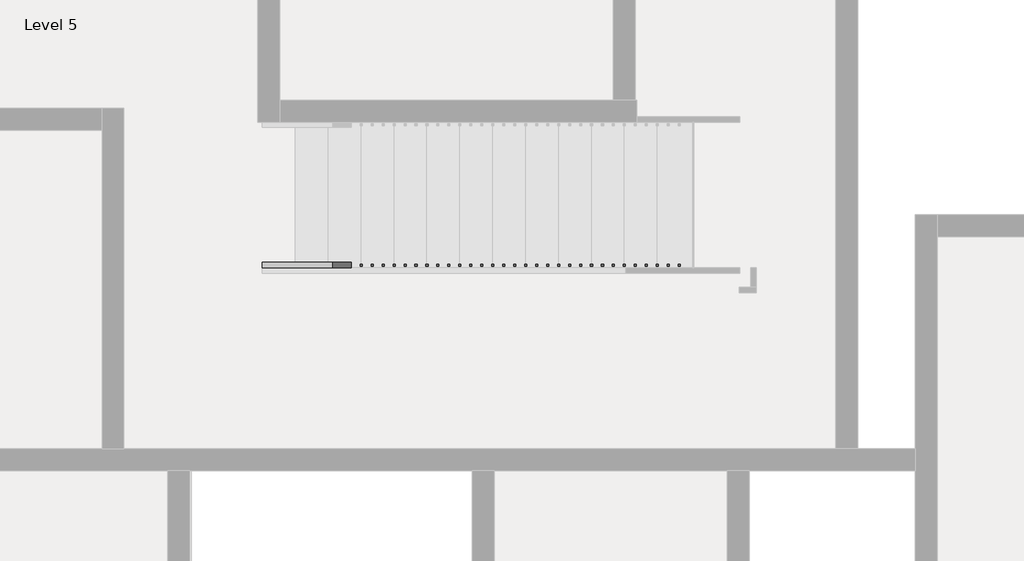
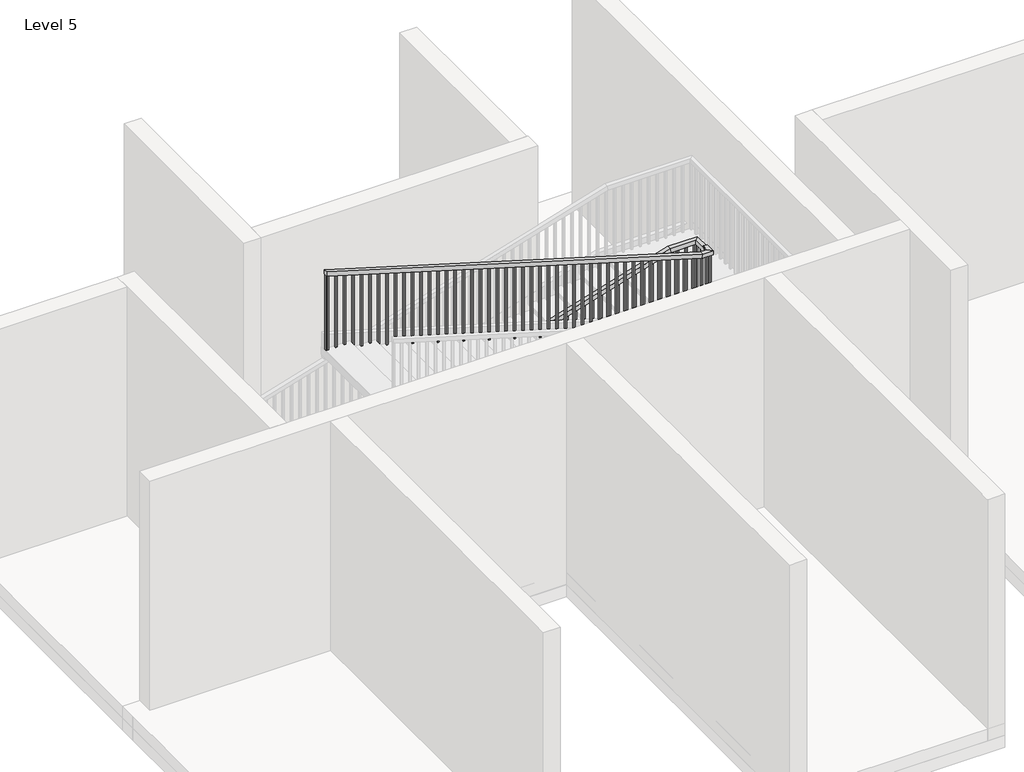
# One storey, part 11 of 14: 1 railing.
"""IFC4 building model written with IfcOpenShell, lengths in millimetres."""

from ifc_helpers import new_model, si_unit, frame, origin, place, context, project, spatial, polyline, outline, extrude, faceted_brep, element, save

model = new_model("IFC4")

# Units and contexts
model_context = context("Model", 3, world=origin())
ifc_project = project(units=[si_unit("LENGTHUNIT", "METRE", prefix="MILLI")], contexts=[model_context])

# Site, building, storey
site = spatial("IfcSite", under=ifc_project)
building = spatial("IfcBuilding", under=site)
storey = spatial("IfcBuildingStorey", under=building, Name="Level 5", Elevation=12192.0)

# Railing
placement = place(None, origin())
element("IfcRailing", 1, ObjectType="Handrail - Rectangular", at=placement, inside=storey, context=model_context, shape_type="SolidModel", body=[
    faceted_brep([(-5254.0891351, 11205.0082924, 13197.84), (-5254.0891351, 11205.0082924, 13144.8032429), (-5254.0891351, 11154.2082924, 13144.8032429), (-5254.0891351, 11154.2082924, 13197.84), (-986.8891351, 11205.0082924, 14478.0), (-979.4332782, 11205.0082924, 14427.2), (-979.4332782, 11154.2082924, 14427.2), (-986.8891351, 11154.2082924, 14478.0), (-631.2891351, 11205.0082924, 14478.0), (-631.2891351, 11205.0082924, 14427.2), (-682.0891351, 11154.2082924, 14427.2), (-682.0891351, 11154.2082924, 14478.0), (-631.2891351, 11001.8082924, 14478.0), (-631.2891351, 10951.0082924, 14427.2), (-682.0891351, 10951.0082924, 14427.2), (-682.0891351, 11001.8082924, 14478.0), (-631.2891351, 11001.8082924, 14500.86), (-631.2891351, 10951.0082924, 14450.06), (-682.0891351, 10951.0082924, 14450.06), (-682.0891351, 11001.8082924, 14500.86), (-631.2891351, 10874.8082924, 14500.86), (-631.2891351, 10874.8082924, 14450.06), (-682.0891351, 10925.6082924, 14450.06), (-682.0891351, 10925.6082924, 14500.86), (-758.2891351, 10874.8082924, 14500.86), (-765.744992, 10874.8082924, 14450.06), (-765.744992, 10925.6082924, 14450.06), (-758.2891351, 10925.6082924, 14500.86), (-5254.0891351, 10874.8082924, 15849.6), (-5254.0891351, 10925.6082924, 15849.6), (-5254.0891351, 10925.6082924, 15796.5632429), (-5254.0891351, 10874.8082924, 15796.5632429)], [[[0, 1, 2, 3]], [[1, 0, 4, 5]], [[2, 1, 5, 6]], [[3, 2, 6, 7]], [[0, 3, 7, 4]], [[5, 4, 8, 9]], [[6, 5, 9, 10]], [[7, 6, 10, 11]], [[4, 7, 11, 8]], [[9, 8, 12, 13]], [[10, 9, 13, 14]], [[11, 10, 14, 15]], [[8, 11, 15, 12]], [[13, 12, 16, 17]], [[14, 13, 17, 18]], [[15, 14, 18, 19]], [[12, 15, 19, 16]], [[17, 16, 20, 21]], [[18, 17, 21, 22]], [[19, 18, 22, 23]], [[16, 19, 23, 20]], [[21, 20, 24, 25]], [[22, 21, 25, 26]], [[23, 22, 26, 27]], [[20, 23, 27, 24]], [[28, 29, 30, 31]], [[25, 24, 28, 31]], [[26, 25, 31, 30]], [[27, 26, 30, 29]], [[24, 27, 29, 28]]]),
    extrude(outline(polyline([(15786.0857429, -5219.1641351), (15791.8007429, -5238.2141351), (14843.76, -5238.2141351), (14843.76, -5219.1641351), (15786.0857429, -5219.1641351)])), frame((0.0, 10890.6832924, 0.0), z_axis=(0.0, 1.0, 0.0), x_axis=(0.0, 0.0, 1.0)), (0.0, 0.0, 1.0), 19.05),
    extrude(outline(polyline([(15755.6057429, -5117.5641351), (15761.3207429, -5136.6141351), (14843.76, -5136.6141351), (14843.76, -5117.5641351), (15755.6057429, -5117.5641351)])), frame((0.0, 10890.6832924, 0.0), z_axis=(0.0, 1.0, 0.0), x_axis=(0.0, 0.0, 1.0)), (0.0, 0.0, 1.0), 19.05),
    extrude(outline(polyline([(15725.1257429, -5015.9641351), (15730.8407429, -5035.0141351), (14843.76, -5035.0141351), (14843.76, -5015.9641351), (15725.1257429, -5015.9641351)])), frame((0.0, 10890.6832924, 0.0), z_axis=(0.0, 1.0, 0.0), x_axis=(0.0, 0.0, 1.0)), (0.0, 0.0, 1.0), 19.05),
    extrude(outline(polyline([(15694.6457429, -4914.3641351), (15700.3607429, -4933.4141351), (14752.32, -4933.4141351), (14752.32, -4914.3641351), (15694.6457429, -4914.3641351)])), frame((0.0, 10890.6832924, 0.0), z_axis=(0.0, 1.0, 0.0), x_axis=(0.0, 0.0, 1.0)), (0.0, 0.0, 1.0), 19.05),
    extrude(outline(polyline([(15664.1657429, -4812.7641351), (15669.8807429, -4831.8141351), (14752.32, -4831.8141351), (14752.32, -4812.7641351), (15664.1657429, -4812.7641351)])), frame((0.0, 10890.6832924, 0.0), z_axis=(0.0, 1.0, 0.0), x_axis=(0.0, 0.0, 1.0)), (0.0, 0.0, 1.0), 19.05),
    extrude(outline(polyline([(15633.6857429, -4711.1641351), (15639.4007429, -4730.2141351), (14752.32, -4730.2141351), (14752.32, -4711.1641351), (15633.6857429, -4711.1641351)])), frame((0.0, 10890.6832924, 0.0), z_axis=(0.0, 1.0, 0.0), x_axis=(0.0, 0.0, 1.0)), (0.0, 0.0, 1.0), 19.05),
    extrude(outline(polyline([(15603.2057429, -4609.5641351), (15608.9207429, -4628.6141351), (14660.88, -4628.6141351), (14660.88, -4609.5641351), (15603.2057429, -4609.5641351)])), frame((0.0, 10890.6832924, 0.0), z_axis=(0.0, 1.0, 0.0), x_axis=(0.0, 0.0, 1.0)), (0.0, 0.0, 1.0), 19.05),
    extrude(outline(polyline([(15572.7257429, -4507.9641351), (15578.4407429, -4527.0141351), (14660.88, -4527.0141351), (14660.88, -4507.9641351), (15572.7257429, -4507.9641351)])), frame((0.0, 10890.6832924, 0.0), z_axis=(0.0, 1.0, 0.0), x_axis=(0.0, 0.0, 1.0)), (0.0, 0.0, 1.0), 19.05),
    extrude(outline(polyline([(15542.2457429, -4406.3641351), (15547.9607429, -4425.4141351), (14660.88, -4425.4141351), (14660.88, -4406.3641351), (15542.2457429, -4406.3641351)])), frame((0.0, 10890.6832924, 0.0), z_axis=(0.0, 1.0, 0.0), x_axis=(0.0, 0.0, 1.0)), (0.0, 0.0, 1.0), 19.05),
    extrude(outline(polyline([(15511.7657429, -4304.7641351), (15517.4807429, -4323.8141351), (14569.44, -4323.8141351), (14569.44, -4304.7641351), (15511.7657429, -4304.7641351)])), frame((0.0, 10890.6832924, 0.0), z_axis=(0.0, 1.0, 0.0), x_axis=(0.0, 0.0, 1.0)), (0.0, 0.0, 1.0), 19.05),
    extrude(outline(polyline([(15481.2857429, -4203.1641351), (15487.0007429, -4222.2141351), (14569.44, -4222.2141351), (14569.44, -4203.1641351), (15481.2857429, -4203.1641351)])), frame((0.0, 10890.6832924, 0.0), z_axis=(0.0, 1.0, 0.0), x_axis=(0.0, 0.0, 1.0)), (0.0, 0.0, 1.0), 19.05),
    extrude(outline(polyline([(15450.8057429, -4101.5641351), (15456.5207429, -4120.6141351), (14569.44, -4120.6141351), (14569.44, -4101.5641351), (15450.8057429, -4101.5641351)])), frame((0.0, 10890.6832924, 0.0), z_axis=(0.0, 1.0, 0.0), x_axis=(0.0, 0.0, 1.0)), (0.0, 0.0, 1.0), 19.05),
    extrude(outline(polyline([(15420.3257429, -3999.9641351), (15426.0407429, -4019.0141351), (14478.0, -4019.0141351), (14478.0, -3999.9641351), (15420.3257429, -3999.9641351)])), frame((0.0, 10890.6832924, 0.0), z_axis=(0.0, 1.0, 0.0), x_axis=(0.0, 0.0, 1.0)), (0.0, 0.0, 1.0), 19.05),
    extrude(outline(polyline([(15389.8457429, -3898.3641351), (15395.5607429, -3917.4141351), (14478.0, -3917.4141351), (14478.0, -3898.3641351), (15389.8457429, -3898.3641351)])), frame((0.0, 10890.6832924, 0.0), z_axis=(0.0, 1.0, 0.0), x_axis=(0.0, 0.0, 1.0)), (0.0, 0.0, 1.0), 19.05),
    extrude(outline(polyline([(15359.3657429, -3796.7641351), (15365.0807429, -3815.8141351), (14478.0, -3815.8141351), (14478.0, -3796.7641351), (15359.3657429, -3796.7641351)])), frame((0.0, 10890.6832924, 0.0), z_axis=(0.0, 1.0, 0.0), x_axis=(0.0, 0.0, 1.0)), (0.0, 0.0, 1.0), 19.05),
    extrude(outline(polyline([(15328.8857429, -3695.1641351), (15334.6007429, -3714.2141351), (14386.56, -3714.2141351), (14386.56, -3695.1641351), (15328.8857429, -3695.1641351)])), frame((0.0, 10890.6832924, 0.0), z_axis=(0.0, 1.0, 0.0), x_axis=(0.0, 0.0, 1.0)), (0.0, 0.0, 1.0), 19.05),
    extrude(outline(polyline([(15298.4057429, -3593.5641351), (15304.1207429, -3612.6141351), (14386.56, -3612.6141351), (14386.56, -3593.5641351), (15298.4057429, -3593.5641351)])), frame((0.0, 10890.6832924, 0.0), z_axis=(0.0, 1.0, 0.0), x_axis=(0.0, 0.0, 1.0)), (0.0, 0.0, 1.0), 19.05),
    extrude(outline(polyline([(15267.9257429, -3491.9641351), (15273.6407429, -3511.0141351), (14386.56, -3511.0141351), (14386.56, -3491.9641351), (15267.9257429, -3491.9641351)])), frame((0.0, 10890.6832924, 0.0), z_axis=(0.0, 1.0, 0.0), x_axis=(0.0, 0.0, 1.0)), (0.0, 0.0, 1.0), 19.05),
    extrude(outline(polyline([(15237.4457429, -3390.3641351), (15243.1607429, -3409.4141351), (14295.12, -3409.4141351), (14295.12, -3390.3641351), (15237.4457429, -3390.3641351)])), frame((0.0, 10890.6832924, 0.0), z_axis=(0.0, 1.0, 0.0), x_axis=(0.0, 0.0, 1.0)), (0.0, 0.0, 1.0), 19.05),
    extrude(outline(polyline([(15206.9657429, -3288.7641351), (15212.6807429, -3307.8141351), (14295.12, -3307.8141351), (14295.12, -3288.7641351), (15206.9657429, -3288.7641351)])), frame((0.0, 10890.6832924, 0.0), z_axis=(0.0, 1.0, 0.0), x_axis=(0.0, 0.0, 1.0)), (0.0, 0.0, 1.0), 19.05),
    extrude(outline(polyline([(15176.4857429, -3187.1641351), (15182.2007429, -3206.2141351), (14295.12, -3206.2141351), (14295.12, -3187.1641351), (15176.4857429, -3187.1641351)])), frame((0.0, 10890.6832924, 0.0), z_axis=(0.0, 1.0, 0.0), x_axis=(0.0, 0.0, 1.0)), (0.0, 0.0, 1.0), 19.05),
    extrude(outline(polyline([(15146.0057429, -3085.5641351), (15151.7207429, -3104.6141351), (14203.68, -3104.6141351), (14203.68, -3085.5641351), (15146.0057429, -3085.5641351)])), frame((0.0, 10890.6832924, 0.0), z_axis=(0.0, 1.0, 0.0), x_axis=(0.0, 0.0, 1.0)), (0.0, 0.0, 1.0), 19.05),
    extrude(outline(polyline([(15115.5257429, -2983.9641351), (15121.2407429, -3003.0141351), (14203.68, -3003.0141351), (14203.68, -2983.9641351), (15115.5257429, -2983.9641351)])), frame((0.0, 10890.6832924, 0.0), z_axis=(0.0, 1.0, 0.0), x_axis=(0.0, 0.0, 1.0)), (0.0, 0.0, 1.0), 19.05),
    extrude(outline(polyline([(15085.0457429, -2882.3641351), (15090.7607429, -2901.4141351), (14203.68, -2901.4141351), (14203.68, -2882.3641351), (15085.0457429, -2882.3641351)])), frame((0.0, 10890.6832924, 0.0), z_axis=(0.0, 1.0, 0.0), x_axis=(0.0, 0.0, 1.0)), (0.0, 0.0, 1.0), 19.05),
    extrude(outline(polyline([(15054.5657429, -2780.7641351), (15060.2807429, -2799.8141351), (14112.24, -2799.8141351), (14112.24, -2780.7641351), (15054.5657429, -2780.7641351)])), frame((0.0, 10890.6832924, 0.0), z_axis=(0.0, 1.0, 0.0), x_axis=(0.0, 0.0, 1.0)), (0.0, 0.0, 1.0), 19.05),
    extrude(outline(polyline([(15024.0857429, -2679.1641351), (15029.8007429, -2698.2141351), (14112.24, -2698.2141351), (14112.24, -2679.1641351), (15024.0857429, -2679.1641351)])), frame((0.0, 10890.6832924, 0.0), z_axis=(0.0, 1.0, 0.0), x_axis=(0.0, 0.0, 1.0)), (0.0, 0.0, 1.0), 19.05),
    extrude(outline(polyline([(14993.6057429, -2577.5641351), (14999.3207429, -2596.6141351), (14112.24, -2596.6141351), (14112.24, -2577.5641351), (14993.6057429, -2577.5641351)])), frame((0.0, 10890.6832924, 0.0), z_axis=(0.0, 1.0, 0.0), x_axis=(0.0, 0.0, 1.0)), (0.0, 0.0, 1.0), 19.05),
    extrude(outline(polyline([(14963.1257429, -2475.9641351), (14968.8407429, -2495.0141351), (14020.8, -2495.0141351), (14020.8, -2475.9641351), (14963.1257429, -2475.9641351)])), frame((0.0, 10890.6832924, 0.0), z_axis=(0.0, 1.0, 0.0), x_axis=(0.0, 0.0, 1.0)), (0.0, 0.0, 1.0), 19.05),
    extrude(outline(polyline([(14932.6457429, -2374.3641351), (14938.3607429, -2393.4141351), (14020.8, -2393.4141351), (14020.8, -2374.3641351), (14932.6457429, -2374.3641351)])), frame((0.0, 10890.6832924, 0.0), z_axis=(0.0, 1.0, 0.0), x_axis=(0.0, 0.0, 1.0)), (0.0, 0.0, 1.0), 19.05),
    extrude(outline(polyline([(14902.1657429, -2272.7641351), (14907.8807429, -2291.8141351), (14020.8, -2291.8141351), (14020.8, -2272.7641351), (14902.1657429, -2272.7641351)])), frame((0.0, 10890.6832924, 0.0), z_axis=(0.0, 1.0, 0.0), x_axis=(0.0, 0.0, 1.0)), (0.0, 0.0, 1.0), 19.05),
    extrude(outline(polyline([(14871.6857429, -2171.1641351), (14877.4007429, -2190.2141351), (13929.36, -2190.2141351), (13929.36, -2171.1641351), (14871.6857429, -2171.1641351)])), frame((0.0, 10890.6832924, 0.0), z_axis=(0.0, 1.0, 0.0), x_axis=(0.0, 0.0, 1.0)), (0.0, 0.0, 1.0), 19.05),
    extrude(outline(polyline([(14841.2057429, -2069.5641351), (14846.9207429, -2088.6141351), (13929.36, -2088.6141351), (13929.36, -2069.5641351), (14841.2057429, -2069.5641351)])), frame((0.0, 10890.6832924, 0.0), z_axis=(0.0, 1.0, 0.0), x_axis=(0.0, 0.0, 1.0)), (0.0, 0.0, 1.0), 19.05),
    extrude(outline(polyline([(14810.7257429, -1967.9641351), (14816.4407429, -1987.0141351), (13929.36, -1987.0141351), (13929.36, -1967.9641351), (14810.7257429, -1967.9641351)])), frame((0.0, 10890.6832924, 0.0), z_axis=(0.0, 1.0, 0.0), x_axis=(0.0, 0.0, 1.0)), (0.0, 0.0, 1.0), 19.05),
    extrude(outline(polyline([(14780.2457429, -1866.3641351), (14785.9607429, -1885.4141351), (13837.92, -1885.4141351), (13837.92, -1866.3641351), (14780.2457429, -1866.3641351)])), frame((0.0, 10890.6832924, 0.0), z_axis=(0.0, 1.0, 0.0), x_axis=(0.0, 0.0, 1.0)), (0.0, 0.0, 1.0), 19.05),
    extrude(outline(polyline([(14749.7657429, -1764.7641351), (14755.4807429, -1783.8141351), (13837.92, -1783.8141351), (13837.92, -1764.7641351), (14749.7657429, -1764.7641351)])), frame((0.0, 10890.6832924, 0.0), z_axis=(0.0, 1.0, 0.0), x_axis=(0.0, 0.0, 1.0)), (0.0, 0.0, 1.0), 19.05),
    extrude(outline(polyline([(14719.2857429, -1663.1641351), (14725.0007429, -1682.2141351), (13837.92, -1682.2141351), (13837.92, -1663.1641351), (14719.2857429, -1663.1641351)])), frame((0.0, 10890.6832924, 0.0), z_axis=(0.0, 1.0, 0.0), x_axis=(0.0, 0.0, 1.0)), (0.0, 0.0, 1.0), 19.05),
    extrude(outline(polyline([(14688.8057429, -1561.5641351), (14694.5207429, -1580.6141351), (13746.48, -1580.6141351), (13746.48, -1561.5641351), (14688.8057429, -1561.5641351)])), frame((0.0, 10890.6832924, 0.0), z_axis=(0.0, 1.0, 0.0), x_axis=(0.0, 0.0, 1.0)), (0.0, 0.0, 1.0), 19.05),
    extrude(outline(polyline([(14658.3257429, -1459.9641351), (14664.0407429, -1479.0141351), (13746.48, -1479.0141351), (13746.48, -1459.9641351), (14658.3257429, -1459.9641351)])), frame((0.0, 10890.6832924, 0.0), z_axis=(0.0, 1.0, 0.0), x_axis=(0.0, 0.0, 1.0)), (0.0, 0.0, 1.0), 19.05),
    extrude(outline(polyline([(14627.8457429, -1358.3641351), (14633.5607429, -1377.4141351), (13746.48, -1377.4141351), (13746.48, -1358.3641351), (14627.8457429, -1358.3641351)])), frame((0.0, 10890.6832924, 0.0), z_axis=(0.0, 1.0, 0.0), x_axis=(0.0, 0.0, 1.0)), (0.0, 0.0, 1.0), 19.05),
    extrude(outline(polyline([(14597.3657429, -1256.7641351), (14603.0807429, -1275.8141351), (13655.04, -1275.8141351), (13655.04, -1256.7641351), (14597.3657429, -1256.7641351)])), frame((0.0, 10890.6832924, 0.0), z_axis=(0.0, 1.0, 0.0), x_axis=(0.0, 0.0, 1.0)), (0.0, 0.0, 1.0), 19.05),
    extrude(outline(polyline([(14566.8857429, -1155.1641351), (14572.6007429, -1174.2141351), (13655.04, -1174.2141351), (13655.04, -1155.1641351), (14566.8857429, -1155.1641351)])), frame((0.0, 10890.6832924, 0.0), z_axis=(0.0, 1.0, 0.0), x_axis=(0.0, 0.0, 1.0)), (0.0, 0.0, 1.0), 19.05),
    extrude(outline(polyline([(14536.4057429, -1053.5641351), (14542.1207429, -1072.6141351), (13655.04, -1072.6141351), (13655.04, -1053.5641351), (14536.4057429, -1053.5641351)])), frame((0.0, 10890.6832924, 0.0), z_axis=(0.0, 1.0, 0.0), x_axis=(0.0, 0.0, 1.0)), (0.0, 0.0, 1.0), 19.05),
    extrude(outline(polyline([(14505.9257429, -951.9641351), (14511.6407429, -971.0141351), (13563.6, -971.0141351), (13563.6, -951.9641351), (14505.9257429, -951.9641351)])), frame((0.0, 10890.6832924, 0.0), z_axis=(0.0, 1.0, 0.0), x_axis=(0.0, 0.0, 1.0)), (0.0, 0.0, 1.0), 19.05),
    extrude(outline(polyline([(14475.4457429, -850.3641351), (14481.1607429, -869.4141351), (13563.6, -869.4141351), (13563.6, -850.3641351), (14475.4457429, -850.3641351)])), frame((0.0, 10890.6832924, 0.0), z_axis=(0.0, 1.0, 0.0), x_axis=(0.0, 0.0, 1.0)), (0.0, 0.0, 1.0), 19.05),
    extrude(outline(polyline([(14444.9657429, -748.7641351), (14450.6807429, -767.8141351), (13563.6, -767.8141351), (13563.6, -748.7641351), (14444.9657429, -748.7641351)])), frame((0.0, 10890.6832924, 0.0), z_axis=(0.0, 1.0, 0.0), x_axis=(0.0, 0.0, 1.0)), (0.0, 0.0, 1.0), 19.05),
    extrude(outline(polyline([(-666.2141351, 10985.9332924), (-647.1641351, 10985.9332924), (-647.1641351, 10966.8832924), (-666.2141351, 10966.8832924), (-666.2141351, 10985.9332924)])), frame((0.0, 0.0, 13563.6), z_axis=(0.0, 0.0, 1.0), x_axis=(1.0, 0.0, 0.0)), (0.0, 0.0, 1.0), 886.46),
    extrude(outline(polyline([(-666.2141351, 11087.5332924), (-647.1641351, 11087.5332924), (-647.1641351, 11068.4832924), (-666.2141351, 11068.4832924), (-666.2141351, 11087.5332924)])), frame((0.0, 0.0, 13563.6), z_axis=(0.0, 0.0, 1.0), x_axis=(1.0, 0.0, 0.0)), (0.0, 0.0, 1.0), 863.6),
    extrude(outline(polyline([(-691.6141351, 11170.0832924), (-691.6141351, 11189.1332924), (-672.5641351, 11189.1332924), (-672.5641351, 11170.0832924), (-691.6141351, 11170.0832924)])), frame((0.0, 0.0, 13563.6), z_axis=(0.0, 0.0, 1.0), x_axis=(1.0, 0.0, 0.0)), (0.0, 0.0, 1.0), 863.6),
    extrude(outline(polyline([(-793.2141351, 11170.0832924), (-793.2141351, 11189.1332924), (-774.1641351, 11189.1332924), (-774.1641351, 11170.0832924), (-793.2141351, 11170.0832924)])), frame((0.0, 0.0, 13563.6), z_axis=(0.0, 0.0, 1.0), x_axis=(1.0, 0.0, 0.0)), (0.0, 0.0, 1.0), 863.6),
    extrude(outline(polyline([(-894.8141351, 11170.0832924), (-894.8141351, 11189.1332924), (-875.7641351, 11189.1332924), (-875.7641351, 11170.0832924), (-894.8141351, 11170.0832924)])), frame((0.0, 0.0, 13563.6), z_axis=(0.0, 0.0, 1.0), x_axis=(1.0, 0.0, 0.0)), (0.0, 0.0, 1.0), 863.6),
    extrude(outline(polyline([(14427.8207429, -977.3641351), (14422.1057429, -996.4141351), (13563.6, -996.4141351), (13563.6, -977.3641351), (14427.8207429, -977.3641351)])), frame((0.0, 11170.0832924, 0.0), z_axis=(0.0, 1.0, 0.0), x_axis=(0.0, 0.0, 1.0)), (0.0, 0.0, 1.0), 19.05),
    extrude(outline(polyline([(14397.3407429, -1078.9641351), (14391.6257429, -1098.0141351), (13472.16, -1098.0141351), (13472.16, -1078.9641351), (14397.3407429, -1078.9641351)])), frame((0.0, 11170.0832924, 0.0), z_axis=(0.0, 1.0, 0.0), x_axis=(0.0, 0.0, 1.0)), (0.0, 0.0, 1.0), 19.05),
    extrude(outline(polyline([(14366.8607429, -1180.5641351), (14361.1457429, -1199.6141351), (13472.16, -1199.6141351), (13472.16, -1180.5641351), (14366.8607429, -1180.5641351)])), frame((0.0, 11170.0832924, 0.0), z_axis=(0.0, 1.0, 0.0), x_axis=(0.0, 0.0, 1.0)), (0.0, 0.0, 1.0), 19.05),
    extrude(outline(polyline([(14336.3807429, -1282.1641351), (14330.6657429, -1301.2141351), (13472.16, -1301.2141351), (13472.16, -1282.1641351), (14336.3807429, -1282.1641351)])), frame((0.0, 11170.0832924, 0.0), z_axis=(0.0, 1.0, 0.0), x_axis=(0.0, 0.0, 1.0)), (0.0, 0.0, 1.0), 19.05),
    extrude(outline(polyline([(14305.9007429, -1383.7641351), (14300.1857429, -1402.8141351), (13380.72, -1402.8141351), (13380.72, -1383.7641351), (14305.9007429, -1383.7641351)])), frame((0.0, 11170.0832924, 0.0), z_axis=(0.0, 1.0, 0.0), x_axis=(0.0, 0.0, 1.0)), (0.0, 0.0, 1.0), 19.05),
    extrude(outline(polyline([(14275.4207429, -1485.3641351), (14269.7057429, -1504.4141351), (13380.72, -1504.4141351), (13380.72, -1485.3641351), (14275.4207429, -1485.3641351)])), frame((0.0, 11170.0832924, 0.0), z_axis=(0.0, 1.0, 0.0), x_axis=(0.0, 0.0, 1.0)), (0.0, 0.0, 1.0), 19.05),
    extrude(outline(polyline([(14244.9407429, -1586.9641351), (14239.2257429, -1606.0141351), (13380.72, -1606.0141351), (13380.72, -1586.9641351), (14244.9407429, -1586.9641351)])), frame((0.0, 11170.0832924, 0.0), z_axis=(0.0, 1.0, 0.0), x_axis=(0.0, 0.0, 1.0)), (0.0, 0.0, 1.0), 19.05),
    extrude(outline(polyline([(14214.4607429, -1688.5641351), (14208.7457429, -1707.6141351), (13289.28, -1707.6141351), (13289.28, -1688.5641351), (14214.4607429, -1688.5641351)])), frame((0.0, 11170.0832924, 0.0), z_axis=(0.0, 1.0, 0.0), x_axis=(0.0, 0.0, 1.0)), (0.0, 0.0, 1.0), 19.05),
    extrude(outline(polyline([(14183.9807429, -1790.1641351), (14178.2657429, -1809.2141351), (13289.28, -1809.2141351), (13289.28, -1790.1641351), (14183.9807429, -1790.1641351)])), frame((0.0, 11170.0832924, 0.0), z_axis=(0.0, 1.0, 0.0), x_axis=(0.0, 0.0, 1.0)), (0.0, 0.0, 1.0), 19.05),
    extrude(outline(polyline([(14153.5007429, -1891.7641351), (14147.7857429, -1910.8141351), (13289.28, -1910.8141351), (13289.28, -1891.7641351), (14153.5007429, -1891.7641351)])), frame((0.0, 11170.0832924, 0.0), z_axis=(0.0, 1.0, 0.0), x_axis=(0.0, 0.0, 1.0)), (0.0, 0.0, 1.0), 19.05),
    extrude(outline(polyline([(14123.0207429, -1993.3641351), (14117.3057429, -2012.4141351), (13197.84, -2012.4141351), (13197.84, -1993.3641351), (14123.0207429, -1993.3641351)])), frame((0.0, 11170.0832924, 0.0), z_axis=(0.0, 1.0, 0.0), x_axis=(0.0, 0.0, 1.0)), (0.0, 0.0, 1.0), 19.05),
    extrude(outline(polyline([(14092.5407429, -2094.9641351), (14086.8257429, -2114.0141351), (13197.84, -2114.0141351), (13197.84, -2094.9641351), (14092.5407429, -2094.9641351)])), frame((0.0, 11170.0832924, 0.0), z_axis=(0.0, 1.0, 0.0), x_axis=(0.0, 0.0, 1.0)), (0.0, 0.0, 1.0), 19.05),
    extrude(outline(polyline([(14062.0607429, -2196.5641351), (14056.3457429, -2215.6141351), (13197.84, -2215.6141351), (13197.84, -2196.5641351), (14062.0607429, -2196.5641351)])), frame((0.0, 11170.0832924, 0.0), z_axis=(0.0, 1.0, 0.0), x_axis=(0.0, 0.0, 1.0)), (0.0, 0.0, 1.0), 19.05),
    extrude(outline(polyline([(14031.5807429, -2298.1641351), (14025.8657429, -2317.2141351), (13106.4, -2317.2141351), (13106.4, -2298.1641351), (14031.5807429, -2298.1641351)])), frame((0.0, 11170.0832924, 0.0), z_axis=(0.0, 1.0, 0.0), x_axis=(0.0, 0.0, 1.0)), (0.0, 0.0, 1.0), 19.05),
    extrude(outline(polyline([(14001.1007429, -2399.7641351), (13995.3857429, -2418.8141351), (13106.4, -2418.8141351), (13106.4, -2399.7641351), (14001.1007429, -2399.7641351)])), frame((0.0, 11170.0832924, 0.0), z_axis=(0.0, 1.0, 0.0), x_axis=(0.0, 0.0, 1.0)), (0.0, 0.0, 1.0), 19.05),
    extrude(outline(polyline([(13970.6207429, -2501.3641351), (13964.9057429, -2520.4141351), (13106.4, -2520.4141351), (13106.4, -2501.3641351), (13970.6207429, -2501.3641351)])), frame((0.0, 11170.0832924, 0.0), z_axis=(0.0, 1.0, 0.0), x_axis=(0.0, 0.0, 1.0)), (0.0, 0.0, 1.0), 19.05),
    extrude(outline(polyline([(13940.1407429, -2602.9641351), (13934.4257429, -2622.0141351), (13014.96, -2622.0141351), (13014.96, -2602.9641351), (13940.1407429, -2602.9641351)])), frame((0.0, 11170.0832924, 0.0), z_axis=(0.0, 1.0, 0.0), x_axis=(0.0, 0.0, 1.0)), (0.0, 0.0, 1.0), 19.05),
    extrude(outline(polyline([(13909.6607429, -2704.5641351), (13903.9457429, -2723.6141351), (13014.96, -2723.6141351), (13014.96, -2704.5641351), (13909.6607429, -2704.5641351)])), frame((0.0, 11170.0832924, 0.0), z_axis=(0.0, 1.0, 0.0), x_axis=(0.0, 0.0, 1.0)), (0.0, 0.0, 1.0), 19.05),
    extrude(outline(polyline([(13879.1807429, -2806.1641351), (13873.4657429, -2825.2141351), (13014.96, -2825.2141351), (13014.96, -2806.1641351), (13879.1807429, -2806.1641351)])), frame((0.0, 11170.0832924, 0.0), z_axis=(0.0, 1.0, 0.0), x_axis=(0.0, 0.0, 1.0)), (0.0, 0.0, 1.0), 19.05),
    extrude(outline(polyline([(13848.7007429, -2907.7641351), (13842.9857429, -2926.8141351), (12923.52, -2926.8141351), (12923.52, -2907.7641351), (13848.7007429, -2907.7641351)])), frame((0.0, 11170.0832924, 0.0), z_axis=(0.0, 1.0, 0.0), x_axis=(0.0, 0.0, 1.0)), (0.0, 0.0, 1.0), 19.05),
    extrude(outline(polyline([(13818.2207429, -3009.3641351), (13812.5057429, -3028.4141351), (12923.52, -3028.4141351), (12923.52, -3009.3641351), (13818.2207429, -3009.3641351)])), frame((0.0, 11170.0832924, 0.0), z_axis=(0.0, 1.0, 0.0), x_axis=(0.0, 0.0, 1.0)), (0.0, 0.0, 1.0), 19.05),
    extrude(outline(polyline([(13787.7407429, -3110.9641351), (13782.0257429, -3130.0141351), (12923.52, -3130.0141351), (12923.52, -3110.9641351), (13787.7407429, -3110.9641351)])), frame((0.0, 11170.0832924, 0.0), z_axis=(0.0, 1.0, 0.0), x_axis=(0.0, 0.0, 1.0)), (0.0, 0.0, 1.0), 19.05),
    extrude(outline(polyline([(13757.2607429, -3212.5641351), (13751.5457429, -3231.6141351), (12832.08, -3231.6141351), (12832.08, -3212.5641351), (13757.2607429, -3212.5641351)])), frame((0.0, 11170.0832924, 0.0), z_axis=(0.0, 1.0, 0.0), x_axis=(0.0, 0.0, 1.0)), (0.0, 0.0, 1.0), 19.05),
    extrude(outline(polyline([(13726.7807429, -3314.1641351), (13721.0657429, -3333.2141351), (12832.08, -3333.2141351), (12832.08, -3314.1641351), (13726.7807429, -3314.1641351)])), frame((0.0, 11170.0832924, 0.0), z_axis=(0.0, 1.0, 0.0), x_axis=(0.0, 0.0, 1.0)), (0.0, 0.0, 1.0), 19.05),
    extrude(outline(polyline([(13696.3007429, -3415.7641351), (13690.5857429, -3434.8141351), (12832.08, -3434.8141351), (12832.08, -3415.7641351), (13696.3007429, -3415.7641351)])), frame((0.0, 11170.0832924, 0.0), z_axis=(0.0, 1.0, 0.0), x_axis=(0.0, 0.0, 1.0)), (0.0, 0.0, 1.0), 19.05),
    extrude(outline(polyline([(13665.8207429, -3517.3641351), (13660.1057429, -3536.4141351), (12740.64, -3536.4141351), (12740.64, -3517.3641351), (13665.8207429, -3517.3641351)])), frame((0.0, 11170.0832924, 0.0), z_axis=(0.0, 1.0, 0.0), x_axis=(0.0, 0.0, 1.0)), (0.0, 0.0, 1.0), 19.05),
    extrude(outline(polyline([(13635.3407429, -3618.9641351), (13629.6257429, -3638.0141351), (12740.64, -3638.0141351), (12740.64, -3618.9641351), (13635.3407429, -3618.9641351)])), frame((0.0, 11170.0832924, 0.0), z_axis=(0.0, 1.0, 0.0), x_axis=(0.0, 0.0, 1.0)), (0.0, 0.0, 1.0), 19.05),
    extrude(outline(polyline([(13604.8607429, -3720.5641351), (13599.1457429, -3739.6141351), (12740.64, -3739.6141351), (12740.64, -3720.5641351), (13604.8607429, -3720.5641351)])), frame((0.0, 11170.0832924, 0.0), z_axis=(0.0, 1.0, 0.0), x_axis=(0.0, 0.0, 1.0)), (0.0, 0.0, 1.0), 19.05),
    extrude(outline(polyline([(13574.3807429, -3822.1641351), (13568.6657429, -3841.2141351), (12649.2, -3841.2141351), (12649.2, -3822.1641351), (13574.3807429, -3822.1641351)])), frame((0.0, 11170.0832924, 0.0), z_axis=(0.0, 1.0, 0.0), x_axis=(0.0, 0.0, 1.0)), (0.0, 0.0, 1.0), 19.05),
    extrude(outline(polyline([(13543.9007429, -3923.7641351), (13538.1857429, -3942.8141351), (12649.2, -3942.8141351), (12649.2, -3923.7641351), (13543.9007429, -3923.7641351)])), frame((0.0, 11170.0832924, 0.0), z_axis=(0.0, 1.0, 0.0), x_axis=(0.0, 0.0, 1.0)), (0.0, 0.0, 1.0), 19.05),
    extrude(outline(polyline([(13513.4207429, -4025.3641351), (13507.7057429, -4044.4141351), (12649.2, -4044.4141351), (12649.2, -4025.3641351), (13513.4207429, -4025.3641351)])), frame((0.0, 11170.0832924, 0.0), z_axis=(0.0, 1.0, 0.0), x_axis=(0.0, 0.0, 1.0)), (0.0, 0.0, 1.0), 19.05),
    extrude(outline(polyline([(13482.9407429, -4126.9641351), (13477.2257429, -4146.0141351), (12557.76, -4146.0141351), (12557.76, -4126.9641351), (13482.9407429, -4126.9641351)])), frame((0.0, 11170.0832924, 0.0), z_axis=(0.0, 1.0, 0.0), x_axis=(0.0, 0.0, 1.0)), (0.0, 0.0, 1.0), 19.05),
    extrude(outline(polyline([(13452.4607429, -4228.5641351), (13446.7457429, -4247.6141351), (12557.76, -4247.6141351), (12557.76, -4228.5641351), (13452.4607429, -4228.5641351)])), frame((0.0, 11170.0832924, 0.0), z_axis=(0.0, 1.0, 0.0), x_axis=(0.0, 0.0, 1.0)), (0.0, 0.0, 1.0), 19.05),
    extrude(outline(polyline([(13421.9807429, -4330.1641351), (13416.2657429, -4349.2141351), (12557.76, -4349.2141351), (12557.76, -4330.1641351), (13421.9807429, -4330.1641351)])), frame((0.0, 11170.0832924, 0.0), z_axis=(0.0, 1.0, 0.0), x_axis=(0.0, 0.0, 1.0)), (0.0, 0.0, 1.0), 19.05),
    extrude(outline(polyline([(13391.5007429, -4431.7641351), (13385.7857429, -4450.8141351), (12466.32, -4450.8141351), (12466.32, -4431.7641351), (13391.5007429, -4431.7641351)])), frame((0.0, 11170.0832924, 0.0), z_axis=(0.0, 1.0, 0.0), x_axis=(0.0, 0.0, 1.0)), (0.0, 0.0, 1.0), 19.05),
    extrude(outline(polyline([(13361.0207429, -4533.3641351), (13355.3057429, -4552.4141351), (12466.32, -4552.4141351), (12466.32, -4533.3641351), (13361.0207429, -4533.3641351)])), frame((0.0, 11170.0832924, 0.0), z_axis=(0.0, 1.0, 0.0), x_axis=(0.0, 0.0, 1.0)), (0.0, 0.0, 1.0), 19.05),
    extrude(outline(polyline([(13330.5407429, -4634.9641351), (13324.8257429, -4654.0141351), (12466.32, -4654.0141351), (12466.32, -4634.9641351), (13330.5407429, -4634.9641351)])), frame((0.0, 11170.0832924, 0.0), z_axis=(0.0, 1.0, 0.0), x_axis=(0.0, 0.0, 1.0)), (0.0, 0.0, 1.0), 19.05),
    extrude(outline(polyline([(13300.0607429, -4736.5641351), (13294.3457429, -4755.6141351), (12374.88, -4755.6141351), (12374.88, -4736.5641351), (13300.0607429, -4736.5641351)])), frame((0.0, 11170.0832924, 0.0), z_axis=(0.0, 1.0, 0.0), x_axis=(0.0, 0.0, 1.0)), (0.0, 0.0, 1.0), 19.05),
    extrude(outline(polyline([(13269.5807429, -4838.1641351), (13263.8657429, -4857.2141351), (12374.88, -4857.2141351), (12374.88, -4838.1641351), (13269.5807429, -4838.1641351)])), frame((0.0, 11170.0832924, 0.0), z_axis=(0.0, 1.0, 0.0), x_axis=(0.0, 0.0, 1.0)), (0.0, 0.0, 1.0), 19.05),
    extrude(outline(polyline([(13239.1007429, -4939.7641351), (13233.3857429, -4958.8141351), (12374.88, -4958.8141351), (12374.88, -4939.7641351), (13239.1007429, -4939.7641351)])), frame((0.0, 11170.0832924, 0.0), z_axis=(0.0, 1.0, 0.0), x_axis=(0.0, 0.0, 1.0)), (0.0, 0.0, 1.0), 19.05),
    extrude(outline(polyline([(13208.6207429, -5041.3641351), (13202.9057429, -5060.4141351), (12283.44, -5060.4141351), (12283.44, -5041.3641351), (13208.6207429, -5041.3641351)])), frame((0.0, 11170.0832924, 0.0), z_axis=(0.0, 1.0, 0.0), x_axis=(0.0, 0.0, 1.0)), (0.0, 0.0, 1.0), 19.05),
    extrude(outline(polyline([(13178.1407429, -5142.9641351), (13172.4257429, -5162.0141351), (12283.44, -5162.0141351), (12283.44, -5142.9641351), (13178.1407429, -5142.9641351)])), frame((0.0, 11170.0832924, 0.0), z_axis=(0.0, 1.0, 0.0), x_axis=(0.0, 0.0, 1.0)), (0.0, 0.0, 1.0), 19.05),
    extrude(outline(polyline([(-666.2141351, 10909.7332924), (-647.1641351, 10909.7332924), (-647.1641351, 10890.6832924), (-666.2141351, 10890.6832924), (-666.2141351, 10909.7332924)])), frame((0.0, 0.0, 13563.6), z_axis=(0.0, 0.0, 1.0), x_axis=(1.0, 0.0, 0.0)), (0.0, 0.0, 1.0), 886.46),
    extrude(outline(polyline([(-666.2141351, 11170.0832924), (-666.2141351, 11189.1332924), (-647.1641351, 11189.1332924), (-647.1641351, 11170.0832924), (-666.2141351, 11170.0832924)])), frame((0.0, 0.0, 13563.6), z_axis=(0.0, 0.0, 1.0), x_axis=(1.0, 0.0, 0.0)), (0.0, 0.0, 1.0), 863.6),
    extrude(outline(polyline([(15790.8482429, -5235.0391351), (15796.5632429, -5254.0891351), (14843.76, -5254.0891351), (14843.76, -5235.0391351), (15790.8482429, -5235.0391351)])), frame((0.0, 10890.6832924, 0.0), z_axis=(0.0, 1.0, 0.0), x_axis=(0.0, 0.0, 1.0)), (0.0, 0.0, 1.0), 19.05),
    extrude(outline(polyline([(13150.5182429, -5235.0391351), (13144.8032429, -5254.0891351), (12283.44, -5254.0891351), (12283.44, -5235.0391351), (13150.5182429, -5235.0391351)])), frame((0.0, 11170.0832924, 0.0), z_axis=(0.0, 1.0, 0.0), x_axis=(0.0, 0.0, 1.0)), (0.0, 0.0, 1.0), 19.05),
])

save(model, "model.ifc")

# Revit data of these elements
# Type "Handrail - Rectangular"
#   Assembly Code = "C2010400"
#   built-in parameter 1008612 = 0.0416667 (stored number, unit not read)
#   built-in parameter 1008611 = 0.0416667 (stored number, unit not read)
#   built-in parameter 1008609 = 0.333333 (stored number, unit not read)
#   built-in parameter 1008604 = 0.166667 (stored number, unit not read)
#   built-in parameter 1008603 = 0.166667 (stored number, unit not read)
#   Railing Height = 3' - 0"
#   built-in parameter 1008630 = 2
#   built-in parameter 1008610 = 2
#   built-in parameter 1008618 = Baluster - Square : 3/4"
# Element 1 (IfcRailing, "Handrail - Rectangular")
#   Phase Created = New Construction
